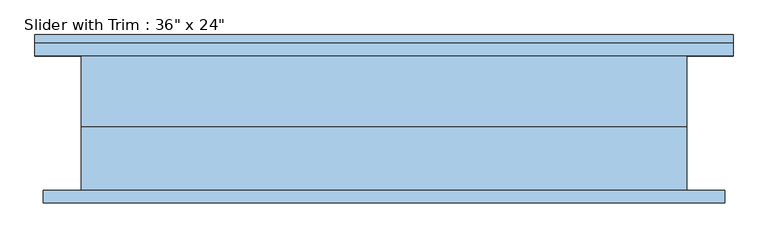
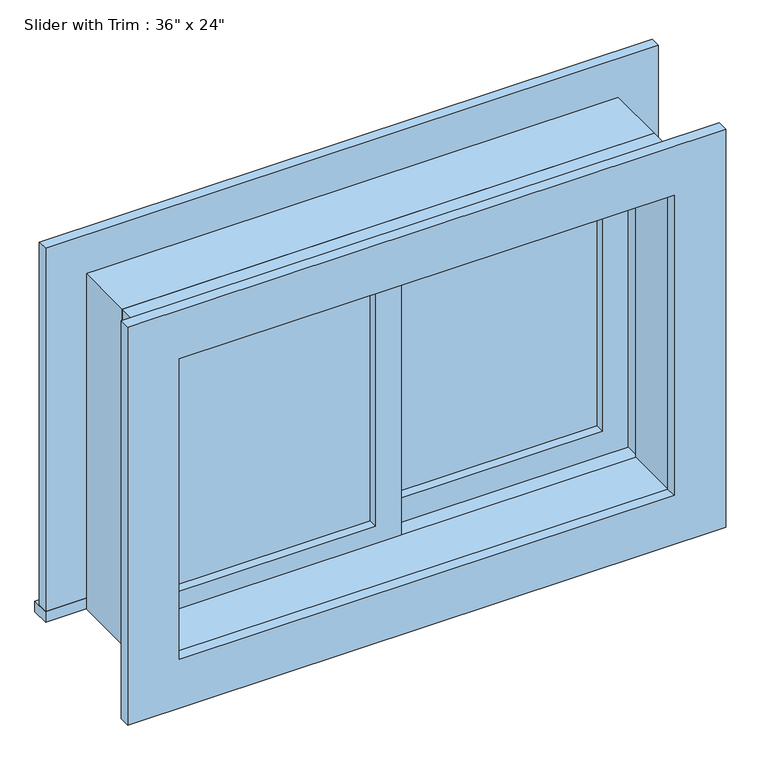
"""IFC4 building model written with IfcOpenShell, lengths in millimetres: window geometry."""

from ifc_helpers import new_model, si_unit, frame, origin, place, context, project, spatial, polyline, outline, extrude, source, transform, mapped, element, save


def window_a4355bb3(model_context):
    return source(origin(), model_context, "Body", "SweptSolid", [
        extrude(outline(polyline([(-393.7, 22.225), (-22.225, 22.225), (-22.225, 9.525), (-393.7, 9.525), (-393.7, 22.225)])), frame((0.0, 0.0, 977.9), z_axis=(0.0, 0.0, 1.0), x_axis=(1.0, 0.0, 0.0)), (0.0, 0.0, 1.0), 482.6),
        extrude(outline(polyline([(1504.95, -438.15), (933.45, -438.15), (933.45, 22.225), (1504.95, 22.225), (1504.95, -438.15)]), holes=[polyline([(1460.5, -393.7), (1460.5, -22.225), (977.9, -22.225), (977.9, -393.7), (1460.5, -393.7)])]), frame((0.0, -6.35, 0.0), z_axis=(0.0, 1.0, 0.0), x_axis=(0.0, 0.0, 1.0)), (0.0, 0.0, 1.0), 44.45),
        extrude(outline(polyline([(-527.05, 133.35), (527.05, 133.35), (527.05, 101.6), (-527.05, 101.6), (-527.05, 133.35)])), frame((0.0, 0.0, 914.4), z_axis=(0.0, 0.0, 1.0), x_axis=(1.0, 0.0, 0.0)), (0.0, 0.0, 1.0), 19.05),
        extrude(outline(polyline([(1504.95, -438.15), (1504.95, 438.15), (933.45, 438.15), (933.45, 527.05), (1593.85, 527.05), (1593.85, -527.05), (933.45, -527.05), (933.45, -438.15), (1504.95, -438.15)])), frame((0.0, 101.6, 0.0), z_axis=(0.0, 1.0, 0.0), x_axis=(0.0, 0.0, 1.0)), (0.0, 0.0, 1.0), 19.05),
        extrude(outline(polyline([(1581.15, 514.35), (1581.15, -514.35), (857.25, -514.35), (857.25, 514.35), (1581.15, 514.35)]), holes=[polyline([(1492.25, 425.45), (946.15, 425.45), (946.15, -425.45), (1492.25, -425.45), (1492.25, 425.45)])]), frame((0.0, -120.65, 0.0), z_axis=(0.0, 1.0, 0.0), x_axis=(0.0, 0.0, 1.0)), (0.0, 0.0, 1.0), 19.05),
        extrude(outline(polyline([(393.7, 53.975), (22.225, 53.975), (22.225, 66.675), (393.7, 66.675), (393.7, 53.975)])), frame((0.0, 0.0, 977.9), z_axis=(0.0, 0.0, 1.0), x_axis=(1.0, 0.0, 0.0)), (0.0, 0.0, 1.0), 482.6),
        extrude(outline(polyline([(1504.95, -22.225), (933.45, -22.225), (933.45, 438.15), (1504.95, 438.15), (1504.95, -22.225)]), holes=[polyline([(1460.5, 22.225), (1460.5, 393.7), (977.9, 393.7), (977.9, 22.225), (1460.5, 22.225)])]), frame((0.0, 38.1, 0.0), z_axis=(0.0, 1.0, 0.0), x_axis=(0.0, 0.0, 1.0)), (0.0, 0.0, 1.0), 44.45),
        extrude(outline(polyline([(1524.0, -457.2), (914.4, -457.2), (914.4, 457.2), (1524.0, 457.2), (1524.0, -457.2)]), holes=[polyline([(1492.25, -425.45), (1492.25, 425.45), (946.15, 425.45), (946.15, -425.45), (1492.25, -425.45)])]), frame((0.0, -101.6, 0.0), z_axis=(0.0, 1.0, 0.0), x_axis=(0.0, 0.0, 1.0)), (0.0, 0.0, 1.0), 95.25),
        extrude(outline(polyline([(1524.0, 457.2), (1524.0, -457.2), (914.4, -457.2), (914.4, 457.2), (1524.0, 457.2)]), holes=[polyline([(1504.95, 438.15), (933.45, 438.15), (933.45, -438.15), (1504.95, -438.15), (1504.95, 438.15)])]), frame((0.0, -6.35, 0.0), z_axis=(0.0, 1.0, 0.0), x_axis=(0.0, 0.0, 1.0)), (0.0, 0.0, 1.0), 107.95),
    ])


if __name__ == "__main__":
    model = new_model("IFC4")
    model_context = context("Model", 3, world=origin())
    ifc_project = project(units=[si_unit("LENGTHUNIT", "METRE", prefix="MILLI")], contexts=[model_context])
    site = spatial("IfcSite", under=ifc_project)
    building = spatial("IfcBuilding", under=site)
    placement = place(None, origin())
    window_shape = window_a4355bb3(model_context)
    element("IfcWindow", 1, ObjectType="Slider with Trim : 36\" x 24\"", at=placement, inside=building, context=model_context, shape_type="MappedRepresentation", body=[
        mapped(window_shape, transform((0.0, 0.0, 0.0), x_axis=(1.0, 0.0, 0.0), y_axis=(0.0, 1.0, 0.0), z_axis=(0.0, 0.0, 1.0))),
    ])
    save(model, "model.ifc")

# Revit data of these elements
# Type "Slider with Trim : 36\" x 24\""
#   Type Mark = "23"
#   Construction Type Id = "GSP4R"
#   Assembly Code = "B2020100"
#   Analytic Construction = "1/8 in Pilkington single glazing"
#   Visual Light Transmittance = 0.9
#   Solar Heat Gain Coefficient = 0.78
#   Heat Transfer Coefficient (U) = 0.6496 BTU/(h·ft²·°F)
#   Height = 2' - 0"
#   Default Sill Height = 3' - 0"
#   Trim Projection - Ext. = 0' - 0 3/4"
#   Trim Projection - Int. = 0' - 0 3/4"
#   Trim Width - Exterior = 0' - 3 1/2"
#   Trim Width - Interior = 0' - 3 1/2"
#   Width = 3' - 0"
#   Window Inset = 0' - 0 3/4"
#   Define Thermal Properties by = 1
#   Glass Pane Material = Glass
#   Sash Material = Sash
#   Trim Exterior Material = Trim
#   Trim Interior Material = Trim
#   Wall Closure = (empty or 0)
# Element 1 (IfcWindow, "Slider with Trim : 36\" x 24\"")
#   Materials on its faces: "Sash", "Trim", "Glass"
# Materials
#   "Glass": class "Glass", colour RGB 0 128 192, transparency 0.75, Description = "Soda Lime Glass", Cost = 0
#   "Sash": class "Wood", colour RGB 224 178 126, transparency 0
#   "Trim": class "Wood", colour RGB 224 178 126, transparency 0
